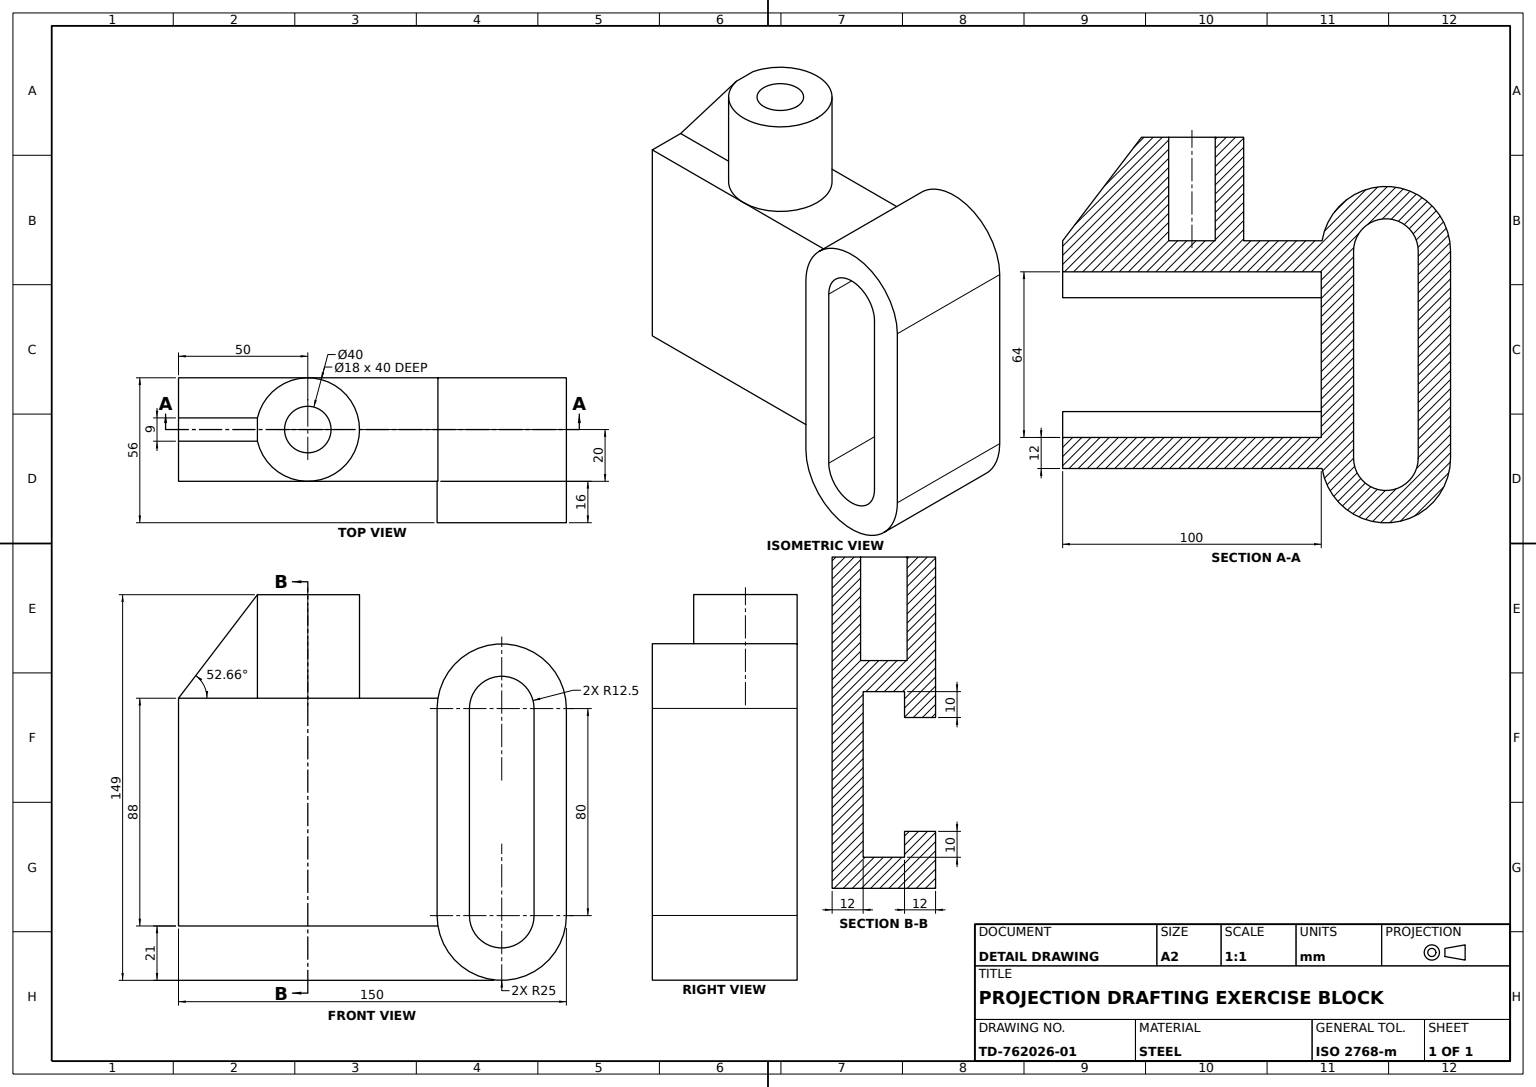
from build123d import *

# Parameters (mm, degrees)
BASE_BLOCK_SKETCH_W         = 40
BASE_BLOCK_SKETCH_H         = 88
BASE_BLOCK_DEPTH            = 50
C_CHANNEL_CUT_DEPTH         = 112.067547015
SLOTTED_LUG_DEPTH           = 40
LUG_START                   = 16
LUG_RIM_DEPTH               = 16
BOSS_CYLINDER_SKETCH_18_R   = 20
BOSS_CYLINDER_SKETCH_18_R_2 = 9
BOSS_CYLINDER_18_DEPTH      = 40
BOSS_EXTENSION_DEPTH        = 40
BOSS_BORE_CUT_DEPTH         = 40
GUSSET_RIB_A_SKETCH_W       = 40
GUSSET_RIB_A_SKETCH_H       = 4
GUSSET_RIB_A_DEPTH          = 10
GUSSET_RIB_B_SKETCH_W       = 40
GUSSET_RIB_B_SKETCH_H       = 4
GUSSET_RIB_B_DEPTH          = 10


with BuildPart() as part:
    # Base Block Sketch → Base Block (new, symmetric)
    with BuildSketch(Plane.XY):
        Rectangle(BASE_BLOCK_SKETCH_W, BASE_BLOCK_SKETCH_H)
    extrude(amount=BASE_BLOCK_DEPTH, both=True)

    # C-Channel Cut Sketch → C-Channel Cut (cut, through all)
    with BuildSketch(Plane.XY.offset(50)):
        Polygon((-20, 22), (-8, 22), (-8, 32), (8, 32), (8, -32), (-8, -32), (-8, -22), (-20, -22), align=None)
    extrude(amount=-C_CHANNEL_CUT_DEPTH, mode=Mode.SUBTRACT)

    # Slotted Lug Sketch → Slotted Lug (add, through all)
    with BuildSketch(Plane(origin=(20, 0, 0), x_dir=(0, 0, -1), z_dir=(1, 0, 0))):
        with BuildLine():
            Line((100, -40), (100, 40))
            ThreePointArc((100, 40), (75, 65), (50, 40))
            Line((50, 40), (50, -40))
            ThreePointArc((50, -40), (75, -65), (100, -40))
        make_face()
        with BuildLine():
            Line((62.5, -40), (62.5, 40))
            ThreePointArc((62.5, 40), (75, 52.5), (87.5, 40))
            Line((87.5, 40), (87.5, -40))
            ThreePointArc((87.5, -40), (75, -52.5), (62.5, -40))
        make_face(mode=Mode.SUBTRACT)
    extrude(amount=-SLOTTED_LUG_DEPTH)

    # Lug Rim Sketch → Lug Rim (add)
    with BuildSketch(Plane(origin=(20, 0, 0), x_dir=(0, 0, -1), z_dir=(1, 0, 0)).offset(LUG_START)):
        with BuildLine():
            Line((50, 40), (50, -40))
            ThreePointArc((50, -40), (75, -65), (100, -40))
            Line((100, -40), (100, 40))
            ThreePointArc((100, 40), (75, 65), (50, 40))
        make_face()
        with BuildLine():
            ThreePointArc((62.5, 40), (75, 52.5), (87.5, 40))
            Line((87.5, 40), (87.5, -40))
            ThreePointArc((87.5, -40), (75, -52.5), (62.5, -40))
            Line((62.5, -40), (62.5, 40))
        make_face(mode=Mode.SUBTRACT)
    extrude(amount=-LUG_RIM_DEPTH)

    # Boss Cylinder Sketch Ø18 → Boss Cylinder Ø18 (add)
    with BuildSketch(Plane(origin=(0, 44, 0), x_dir=(1, 0, 0), z_dir=(0, 1, 0))):
        with Locations(Location((0, 0, 0), (0, 0, 180))):
            Circle(BOSS_CYLINDER_SKETCH_18_R)
        with Locations(Location((0, 0, 0), (0, 0, 270))):
            Circle(BOSS_CYLINDER_SKETCH_18_R_2, mode=Mode.SUBTRACT)
    extrude(amount=BOSS_CYLINDER_18_DEPTH)

    # Boss Extension Sketch → Boss Extension (add)
    with BuildSketch(Plane(origin=(0, 44, 0), x_dir=(1, 0, 0), z_dir=(0, 1, 0))):
        with BuildLine():
            Line((-4.5, -19.48717527), (-4.5, -50))
            Line((-4.5, -50), (4.5, -50))
            Line((4.5, -50), (4.5, -19.48717527))
            ThreePointArc((4.5, -19.48717527), (0, -20), (-4.5, -19.48717527))
        make_face()
    extrude(amount=BOSS_EXTENSION_DEPTH)

    # Boss Bore Sketch → Boss Bore Cut (cut)
    with BuildSketch(Plane.ZY.offset(4.5)):
        Polygon((19.48717527, 84), (50, 44), (50, 84), align=None)
    extrude(amount=-BOSS_BORE_CUT_DEPTH, mode=Mode.SUBTRACT)

    # Gusset Rib A Sketch → Gusset Rib A (add)
    with BuildSketch(Plane(origin=(0, 0, -50), x_dir=(-1, 0, 0), z_dir=(0, 0, -1))):
        with Locations((0, 42)):
            Rectangle(GUSSET_RIB_A_SKETCH_W, GUSSET_RIB_A_SKETCH_H)
    extrude(amount=GUSSET_RIB_A_DEPTH)

    # Gusset Rib B Sketch → Gusset Rib B (add)
    with BuildSketch(Plane(origin=(0, 0, -50), x_dir=(-1, 0, 0), z_dir=(0, 0, -1))):
        with Locations((0, -42)):
            Rectangle(GUSSET_RIB_B_SKETCH_W, GUSSET_RIB_B_SKETCH_H)
    extrude(amount=GUSSET_RIB_B_DEPTH)


solid = part.part
